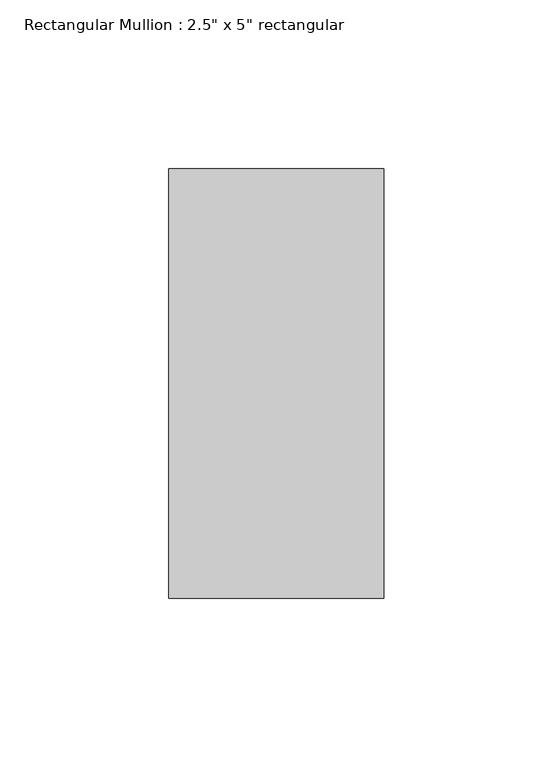
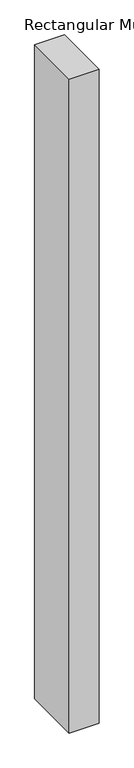
"""IFC4 building model written with IfcOpenShell, lengths in millimetres: member geometry."""

from ifc_helpers import new_model, si_unit, frame, origin, place, context, project, spatial, polyline, outline, extrude, source, transform, mapped, element, save


def member_03ac5645(model_context):
    return source(origin(), model_context, "Body", "SweptSolid", [
        extrude(outline(polyline([(0.0, 63.5), (0.0, -63.5), (-63.5, -63.5), (-63.5, 63.5), (0.0, 63.5)])), frame((0.0, 0.0, -1471.9817095), z_axis=(0.0, 0.0, 1.0), x_axis=(1.0, 0.0, 0.0)), (0.0, 0.0, 1.0), 1471.9817095),
    ])


if __name__ == "__main__":
    model = new_model("IFC4")
    model_context = context("Model", 3, world=origin())
    ifc_project = project(units=[si_unit("LENGTHUNIT", "METRE", prefix="MILLI")], contexts=[model_context])
    site = spatial("IfcSite", under=ifc_project)
    building = spatial("IfcBuilding", under=site)
    placement = place(None, origin())
    member_shape = member_03ac5645(model_context)
    element("IfcMember", 1, ObjectType="Rectangular Mullion : 2.5\" x 5\" rectangular", at=placement, inside=building, context=model_context, shape_type="MappedRepresentation", body=[
        mapped(member_shape, transform((0.0, 0.0, 0.0), x_axis=(1.0, 0.0, 0.0), y_axis=(0.0, 1.0, 0.0), z_axis=(0.0, 0.0, 1.0))),
    ])
    save(model, "model.ifc")

# Revit data of these elements
# Type "Rectangular Mullion : 2.5\" x 5\" rectangular"
#   built-in parameter 1007304 = 0.416667 (stored number, unit not read)
#   built-in parameter 1007301 = 0.104167 (stored number, unit not read)
#   built-in parameter 1007300 = 0.104167 (stored number, unit not read)
# Element 1 (IfcMember, "Rectangular Mullion : 2.5\" x 5\" rectangular")
#   Materials on its faces: "Aluminum"
# Materials
#   "Aluminum": class "Metal", colour RGB 247 247 247, transparency 0, Description = "Aluminum 6061", Cost = 0
